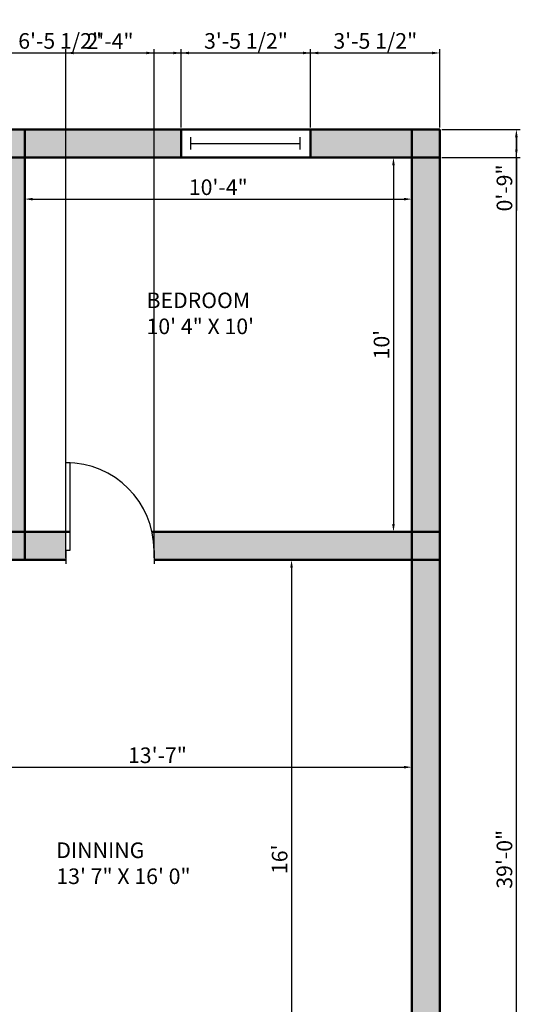
# Model space of a CAD drawing. Units: millimetres. Extents: x 2784 to 3697, y 603 to 1406.
# Tile 10 of 10: x 3537 to 3697, y 953 to 1268. Entities that reach past the tile are written whole.
import ezdxf

# ---------------------------------------------------------------- set-up
doc = ezdxf.new("R2010")
doc.units = ezdxf.units.MM
for name, color, linetype, lineweight in [('A-ANNO-DIMS', 140, 'Continuous', 18), ('A-AREA-IDEN', 150, 'Continuous', 25), ('A-DOOR', 10, 'Continuous', 25), ('A-GLAZ', 30, 'Continuous', 25), ('A-WALL', 2, 'Continuous', 50), ('A-WALL-PATT', 8, 'Continuous', 13)]:
    doc.layers.add(name, color=color, linetype=linetype, lineweight=lineweight)
doc.styles.get("Standard").update_dxf_attribs({"font": 'arial.ttf'})
doc.dimstyles.new('ISO-25', dxfattribs={"dimtxt": 5, "dimasz": 2.5, "dimexe": 1.25, "dimexo": 0.625, "dimtad": 1, "dimdec": 0, "dimlunit": 3, "dimtxsty": 'Standard', "dimcen": 2.5, "dimadec": 0, "dimazin": 0, "dimtfac": 1, "dimtdec": 0, "dimtmove": 0, "dimatfit": 3, "dimfxl": 1, "dimarcsym": 0})

# ---------------------------------------------------------------- blocks, each defined once
blk = doc.blocks.new('*U2')
for p, q in [((0, 0), (0, -6)), ((40, 0), (40, -6))]:
    blk.add_line(p, q)
blk.add_lwpolyline([(0, 0), (0, 40), (1.75, 40), (1.75, 0)], close=True)
blk.add_arc((0, 0), 40, 0, 90)
blk = doc.blocks.new('*U38')
for p, q in [((0, 4), (0, 0)), ((36, 4), (36, 0)), ((0, 2), (36, 2))]:
    blk.add_line(p, q)
blk = doc.blocks.new('*D43')
at = {"layer": 'A-ANNO-DIMS', "color": 0, "lineweight": -2, "transparency": 16777216}
for p, q in [((3661.6, 1224.28), (3655.11, 1224.28)), ((3656.36, 1221.78), (3656.36, 1106.78)), ((3661.6, 1104.28), (3655.11, 1104.28))]:
    blk.add_line(p, q, dxfattribs=at)
at = {"layer": 'A-ANNO-DIMS', "color": 0, "transparency": 16777216}
for points in [[(3655.94, 1221.78), (3656.77, 1221.78), (3656.36, 1224.28)], [(3655.94, 1106.78), (3656.77, 1106.78), (3656.36, 1104.28)]]:
    blk.add_solid(points, dxfattribs=at)
at = {"layer": 'Defpoints', "color": 0, "transparency": 16777216}
for p in [(3662.23, 1224.28), (3656.36, 1104.28), (3662.23, 1104.28)]:
    blk.add_point(p, dxfattribs=at)
at = {"layer": 'A-ANNO-DIMS', "color": 0, "transparency": 16777216, "insert": (3653.18, 1164.28), "char_height": 5, "attachment_point": 5, "rotation": 90}
blk.add_mtext("10'", dxfattribs=at)
blk = doc.blocks.new('*D44')
at = {"layer": 'A-ANNO-DIMS', "color": 0, "lineweight": -2, "transparency": 16777216}
for p, q in [((3538.23, 1211.55), (3538.23, 1212.18)), ((3662.23, 1211.55), (3662.23, 1212.18)), ((3540.73, 1210.93), (3659.73, 1210.93))]:
    blk.add_line(p, q, dxfattribs=at)
at = {"layer": 'A-ANNO-DIMS', "color": 0, "transparency": 16777216}
for points in [[(3540.73, 1211.34), (3540.73, 1210.51), (3538.23, 1210.93)], [(3659.73, 1211.34), (3659.73, 1210.51), (3662.23, 1210.93)]]:
    blk.add_solid(points, dxfattribs=at)
at = {"layer": 'Defpoints', "color": 0, "transparency": 16777216}
for p in [(3538.23, 1210.93), (3662.23, 1210.93), (3662.23, 1210.93)]:
    blk.add_point(p, dxfattribs=at)
at = {"layer": 'A-ANNO-DIMS', "color": 0, "transparency": 16777216, "insert": (3600.23, 1214.1), "char_height": 5, "attachment_point": 5}
blk.add_mtext('10\'-4"', dxfattribs=at)
blk = doc.blocks.new('*D58')
at = {"layer": 'A-ANNO-DIMS', "color": 0, "lineweight": -2, "transparency": 16777216}
for p, q in [((3624.82, 1095.28), (3622.46, 1095.28)), ((3623.71, 1092.78), (3623.71, 905.81)), ((3624.82, 903.31), (3622.46, 903.31))]:
    blk.add_line(p, q, dxfattribs=at)
at = {"layer": 'A-ANNO-DIMS', "color": 0, "transparency": 16777216}
for points in [[(3623.29, 1092.78), (3624.12, 1092.78), (3623.71, 1095.28)], [(3623.29, 905.81), (3624.12, 905.81), (3623.71, 903.31)]]:
    blk.add_solid(points, dxfattribs=at)
at = {"layer": 'Defpoints', "color": 0, "transparency": 16777216}
for p in [(3625.44, 1095.28), (3623.71, 903.31), (3625.44, 903.31)]:
    blk.add_point(p, dxfattribs=at)
at = {"layer": 'A-ANNO-DIMS', "color": 0, "transparency": 16777216, "insert": (3620.53, 999.3), "char_height": 5, "attachment_point": 5, "rotation": 90}
blk.add_mtext("16'", dxfattribs=at)
blk = doc.blocks.new('*D59')
at = {"layer": 'A-ANNO-DIMS', "color": 0, "lineweight": -2, "transparency": 16777216}
for p, q in [((3499.23, 1028.23), (3499.23, 1030.07)), ((3662.23, 1028.23), (3662.23, 1030.07)), ((3501.73, 1028.82), (3659.73, 1028.82))]:
    blk.add_line(p, q, dxfattribs=at)
at = {"layer": 'A-ANNO-DIMS', "color": 0, "transparency": 16777216}
for points in [[(3501.73, 1029.23), (3501.73, 1028.4), (3499.23, 1028.82)], [(3659.73, 1029.23), (3659.73, 1028.4), (3662.23, 1028.82)]]:
    blk.add_solid(points, dxfattribs=at)
at = {"layer": 'Defpoints', "color": 0, "transparency": 16777216}
for p in [(3499.23, 1027.6), (3662.23, 1028.82), (3662.23, 1027.6)]:
    blk.add_point(p, dxfattribs=at)
at = {"layer": 'A-ANNO-DIMS', "color": 0, "transparency": 16777216, "insert": (3580.73, 1032), "char_height": 5, "attachment_point": 5}
blk.add_mtext('13\'-7"', dxfattribs=at)
blk = doc.blocks.new('*D110')
at = {"layer": 'A-ANNO-DIMS', "color": 0, "lineweight": -2, "transparency": 16777216}
for p, q in [((3307.23, 1233.91), (3307.23, 1259.03)), ((3309.73, 1257.78), (3668.73, 1257.78)), ((3671.23, 1233.91), (3671.23, 1259.03))]:
    blk.add_line(p, q, dxfattribs=at)
at = {"layer": 'A-ANNO-DIMS', "color": 0, "transparency": 16777216}
for points in [[(3309.73, 1258.2), (3309.73, 1257.36), (3307.23, 1257.78)], [(3668.73, 1258.2), (3668.73, 1257.36), (3671.23, 1257.78)]]:
    blk.add_solid(points, dxfattribs=at)
at = {"layer": 'Defpoints', "color": 0, "transparency": 16777216}
for p in [(3671.23, 1257.78), (3307.23, 1233.28), (3671.23, 1233.28)]:
    blk.add_point(p, dxfattribs=at)
at = {"layer": 'A-ANNO-DIMS', "color": 0, "transparency": 16777216, "insert": (3489.23, 1260.96), "char_height": 5, "attachment_point": 5}
blk.add_mtext('30\'-4"', dxfattribs=at)
blk = doc.blocks.new('*D115')
at = {"layer": 'A-ANNO-DIMS', "color": 0, "lineweight": -2, "transparency": 16777216}
for p, q in [((3510.77, 1233.91), (3510.77, 1259.03)), ((3513.27, 1257.78), (3585.87, 1257.78)), ((3588.37, 1233.91), (3588.37, 1259.03))]:
    blk.add_line(p, q, dxfattribs=at)
at = {"layer": 'A-ANNO-DIMS', "color": 0, "transparency": 16777216}
for points in [[(3513.27, 1258.2), (3513.27, 1257.36), (3510.77, 1257.78)], [(3585.87, 1258.2), (3585.87, 1257.36), (3588.37, 1257.78)]]:
    blk.add_solid(points, dxfattribs=at)
at = {"layer": 'Defpoints', "color": 0, "transparency": 16777216}
for p in [(3588.37, 1257.78), (3510.77, 1233.28), (3588.37, 1233.28)]:
    blk.add_point(p, dxfattribs=at)
at = {"layer": 'A-ANNO-DIMS', "color": 0, "transparency": 16777216, "insert": (3549.57, 1260.99), "char_height": 5, "attachment_point": 5}
blk.add_mtext('6\'-5 1/2"', dxfattribs=at)
blk = doc.blocks.new('*D116')
at = {"layer": 'A-ANNO-DIMS', "color": 0, "lineweight": -2, "transparency": 16777216}
for p, q in [((3588.37, 1233.91), (3588.37, 1259.03)), ((3590.87, 1257.78), (3627.32, 1257.78)), ((3629.82, 1233.91), (3629.82, 1259.03))]:
    blk.add_line(p, q, dxfattribs=at)
at = {"layer": 'A-ANNO-DIMS', "color": 0, "transparency": 16777216}
for points in [[(3590.87, 1258.2), (3590.87, 1257.36), (3588.37, 1257.78)], [(3627.32, 1258.2), (3627.32, 1257.36), (3629.82, 1257.78)]]:
    blk.add_solid(points, dxfattribs=at)
at = {"layer": 'Defpoints', "color": 0, "transparency": 16777216}
for p in [(3629.82, 1257.78), (3588.37, 1233.28), (3629.82, 1233.28)]:
    blk.add_point(p, dxfattribs=at)
at = {"layer": 'A-ANNO-DIMS', "color": 0, "transparency": 16777216, "insert": (3609.1, 1260.99), "char_height": 5, "attachment_point": 5}
blk.add_mtext('3\'-5 1/2"', dxfattribs=at)
blk = doc.blocks.new('*D117')
at = {"layer": 'A-ANNO-DIMS', "color": 0, "lineweight": -2, "transparency": 16777216}
for p, q in [((3629.82, 1233.91), (3629.82, 1259.03)), ((3632.32, 1257.78), (3668.73, 1257.78)), ((3671.23, 1233.91), (3671.23, 1259.03))]:
    blk.add_line(p, q, dxfattribs=at)
at = {"layer": 'A-ANNO-DIMS', "color": 0, "transparency": 16777216}
for points in [[(3632.32, 1258.2), (3632.32, 1257.36), (3629.82, 1257.78)], [(3668.73, 1258.2), (3668.73, 1257.36), (3671.23, 1257.78)]]:
    blk.add_solid(points, dxfattribs=at)
at = {"layer": 'Defpoints', "color": 0, "transparency": 16777216}
for p in [(3671.23, 1257.78), (3629.82, 1233.28), (3671.23, 1233.28)]:
    blk.add_point(p, dxfattribs=at)
at = {"layer": 'A-ANNO-DIMS', "color": 0, "transparency": 16777216, "insert": (3650.53, 1260.99), "char_height": 5, "attachment_point": 5}
blk.add_mtext('3\'-5 1/2"', dxfattribs=at)
blk = doc.blocks.new('*D130')
at = {"layer": 'A-ANNO-DIMS', "color": 0, "lineweight": -2, "transparency": 16777216}
for p, q in [((3671.85, 1233.28), (3696.98, 1233.28)), ((3695.73, 767.81), (3695.73, 1230.78)), ((3671.85, 765.31), (3696.98, 765.31))]:
    blk.add_line(p, q, dxfattribs=at)
at = {"layer": 'A-ANNO-DIMS', "color": 0, "transparency": 16777216}
for points in [[(3695.31, 1230.78), (3696.14, 1230.78), (3695.73, 1233.28)], [(3695.31, 767.81), (3696.14, 767.81), (3695.73, 765.31)]]:
    blk.add_solid(points, dxfattribs=at)
at = {"layer": 'Defpoints', "color": 0, "transparency": 16777216}
for p in [(3671.23, 1233.28), (3695.73, 1233.28), (3671.23, 765.31)]:
    blk.add_point(p, dxfattribs=at)
at = {"layer": 'A-ANNO-DIMS', "color": 0, "transparency": 16777216, "insert": (3692.55, 999.3), "char_height": 5, "attachment_point": 5, "rotation": 90}
blk.add_mtext('39\'-0"', dxfattribs=at)
blk = doc.blocks.new('*D131')
at = {"layer": 'A-ANNO-DIMS', "color": 0, "lineweight": -2, "transparency": 16777216}
for p, q in [((3671.85, 1233.28), (3696.98, 1233.28)), ((3695.73, 1230.78), (3695.73, 1226.78)), ((3671.85, 1224.28), (3696.98, 1224.28)), ((3695.73, 1224.28), (3695.73, 1207.24))]:
    blk.add_line(p, q, dxfattribs=at)
at = {"layer": 'A-ANNO-DIMS', "color": 0, "transparency": 16777216}
for points in [[(3695.31, 1230.78), (3696.14, 1230.78), (3695.73, 1233.28)], [(3695.31, 1226.78), (3696.14, 1226.78), (3695.73, 1224.28)]]:
    blk.add_solid(points, dxfattribs=at)
at = {"layer": 'Defpoints', "color": 0, "transparency": 16777216}
for p in [(3671.23, 1233.28), (3671.23, 1224.28), (3695.73, 1224.28)]:
    blk.add_point(p, dxfattribs=at)
at = {"layer": 'A-ANNO-DIMS', "color": 0, "transparency": 16777216, "insert": (3692.55, 1214.51), "char_height": 5, "attachment_point": 5, "rotation": 90}
blk.add_mtext('0\'-9"', dxfattribs=at)
blk = doc.blocks.new('*D134')
at = {"layer": 'A-ANNO-DIMS', "color": 0, "lineweight": -2, "transparency": 16777216}
for p, q in [((3551.44, 1095.91), (3551.44, 1259.03)), ((3553.94, 1257.78), (3577.16, 1257.78)), ((3579.66, 1095.91), (3579.66, 1259.03))]:
    blk.add_line(p, q, dxfattribs=at)
at = {"layer": 'A-ANNO-DIMS', "color": 0, "transparency": 16777216}
for points in [[(3553.94, 1258.2), (3553.94, 1257.36), (3551.44, 1257.78)], [(3577.16, 1258.2), (3577.16, 1257.36), (3579.66, 1257.78)]]:
    blk.add_solid(points, dxfattribs=at)
at = {"layer": 'Defpoints', "color": 0, "transparency": 16777216}
for p in [(3579.66, 1257.78), (3551.44, 1095.28), (3579.66, 1095.28)]:
    blk.add_point(p, dxfattribs=at)
at = {"layer": 'A-ANNO-DIMS', "color": 0, "transparency": 16777216, "insert": (3565.55, 1260.92), "char_height": 5, "attachment_point": 5}
blk.add_mtext('2\'-4"', dxfattribs=at)

msp = doc.modelspace()

# ---------------------------------------------------------------- hatches: boundary and pattern name
at = {"layer": 'A-WALL-PATT'}
h = msp.add_hatch(color=256, dxfattribs=at)
h.dxf.hatch_style = 1
h.paths.add_polyline_path([(3316.23, 1224.28), (3307.23, 1224.28), (3307.23, 1104.28), (3316.23, 1104.28)])
h.paths.add_polyline_path([(3316.23, 1233.28), (3307.23, 1233.28), (3307.23, 1224.28), (3316.23, 1224.28)])
h.paths.add_polyline_path([(3363.37, 1233.28), (3316.23, 1233.28), (3316.23, 1224.28), (3363.37, 1224.28)])
h.paths.add_polyline_path([(3460.23, 1233.28), (3405.1, 1233.28), (3405.1, 1224.28), (3460.23, 1224.28)])
h.paths.add_polyline_path([(3469.23, 1233.28), (3460.23, 1233.28), (3460.23, 1224.28), (3469.23, 1224.28)])
h.paths.add_polyline_path([(3469.23, 1224.28), (3460.23, 1224.28), (3460.23, 1104.28), (3469.23, 1104.28)])
h.paths.add_polyline_path([(3469.23, 1104.28), (3460.23, 1104.28), (3460.23, 1095.28), (3469.23, 1095.28)])
h.paths.add_polyline_path([(3460.23, 1104.28), (3444.39, 1104.28), (3444.39, 1097.52), (3444.39, 1095.28), (3460.23, 1095.28)])
h.paths.add_polyline_path([(3409.23, 1095.28), (3400.23, 1095.28), (3400.23, 1066.17, -0.119943), (3407.82, 1068.02), (3409.23, 1068.02)])
h.paths.add_polyline_path([(3409.23, 1104.28), (3400.23, 1104.28), (3400.23, 1095.28), (3409.23, 1095.28)])
h.paths.add_polyline_path([(3400.23, 1104.28), (3316.23, 1104.28), (3316.23, 1095.28), (3400.23, 1095.28)])
h.paths.add_polyline_path([(3316.23, 1104.28), (3307.23, 1104.28), (3307.23, 1095.28), (3316.23, 1095.28)])
h.paths.add_polyline_path([(3316.23, 1095.28), (3307.23, 1095.28), (3307.23, 1083.49), (3316.23, 1083.49)])
h.paths.add_polyline_path([(3416.17, 1097.52, -0.060509), (3416.99, 1104.28), (3409.23, 1104.28), (3409.23, 1095.28), (3416.17, 1095.28)])
h.paths.add_polyline_path([(3538.23, 1224.28), (3529.23, 1224.28), (3529.23, 1104.28), (3538.23, 1104.28)])
h.paths.add_polyline_path([(3538.23, 1233.28), (3529.23, 1233.28), (3529.23, 1224.28), (3538.23, 1224.28)])
h.paths.add_polyline_path([(3529.23, 1233.28), (3510.77, 1233.28), (3510.77, 1224.28), (3529.23, 1224.28)])
h.paths.add_polyline_path([(3483.89, 1233.28), (3469.23, 1233.28), (3469.23, 1224.28), (3483.89, 1224.28)])
h.paths.add_polyline_path([(3662.23, 1233.28), (3629.82, 1233.28), (3629.82, 1224.28), (3662.23, 1224.28)])
h.paths.add_polyline_path([(3671.23, 1233.28), (3662.23, 1233.28), (3662.23, 1224.28), (3671.23, 1224.28)])
h.paths.add_polyline_path([(3671.23, 1224.28), (3662.23, 1224.28), (3662.23, 1104.28), (3671.23, 1104.28)])
h.paths.add_polyline_path([(3588.37, 1233.28), (3538.23, 1233.28), (3538.23, 1224.28), (3588.37, 1224.28)])
h.paths.add_polyline_path([(3662.23, 1104.28), (3579.01, 1104.28, -0.053945), (3579.66, 1098.24), (3579.66, 1095.28), (3662.23, 1095.28)])
h.paths.add_polyline_path([(3671.23, 1104.28), (3662.23, 1104.28), (3662.23, 1095.28), (3671.23, 1095.28)])
h.paths.add_polyline_path([(3551.44, 1104.28), (3538.23, 1104.28), (3538.23, 1095.28), (3551.44, 1095.28), (3551.44, 1098.24)])
h.paths.add_polyline_path([(3538.23, 1104.28), (3529.23, 1104.28), (3529.23, 1095.28), (3538.23, 1095.28)])
h.paths.add_polyline_path([(3671.23, 1095.28), (3662.23, 1095.28), (3662.23, 903.31), (3671.23, 903.31)])
h.paths.add_polyline_path([(3316.23, 985.84), (3307.23, 985.84), (3307.23, 932.57), (3316.23, 932.57)])
h.paths.add_polyline_path([(3316.23, 1041.28), (3307.23, 1041.28), (3307.23, 1012.14), (3316.23, 1012.14)])
h.paths.add_polyline_path([(3316.23, 1050.28), (3307.23, 1050.28), (3307.23, 1041.28), (3316.23, 1041.28)])
h.paths.add_polyline_path([(3400.23, 1050.28), (3316.23, 1050.28), (3316.23, 1041.28), (3400.23, 1041.28)])
h.paths.add_polyline_path([(3316.23, 1059.19), (3307.23, 1059.19), (3307.23, 1050.28), (3316.23, 1050.28)])
h.paths.add_polyline_path([(3316.23, 908.17), (3307.23, 908.17), (3307.23, 774.31), (3316.23, 774.31)])
h.paths.add_polyline_path([(3316.23, 774.31), (3307.23, 774.31), (3307.23, 765.31), (3316.23, 765.31)])
h.paths.add_polyline_path([(3372.55, 774.31), (3316.23, 774.31), (3316.23, 765.31), (3372.55, 765.31)])
h.paths.add_polyline_path([(3505.23, 774.31), (3416.56, 774.31), (3416.56, 765.31), (3505.23, 765.31)])
h.paths.add_polyline_path([(3568.83, 774.31), (3514.23, 774.31), (3514.23, 765.31), (3568.83, 765.31)])
h.paths.add_polyline_path([(3514.23, 774.31), (3505.23, 774.31), (3505.23, 765.31), (3514.23, 765.31)])
h.paths.add_polyline_path([(3514.23, 894.31), (3505.23, 894.31), (3505.23, 774.31), (3514.23, 774.31)])
h.paths.add_polyline_path([(3514.23, 903.31), (3505.23, 903.31), (3505.23, 894.31), (3514.23, 894.31)])
h.paths.add_polyline_path([(3473.23, 948.31), (3464.23, 948.31), (3464.23, 903.31), (3473.23, 903.31)])
h.paths.add_polyline_path([(3473.23, 903.31), (3464.23, 903.31), (3464.23, 894.31), (3473.23, 894.31)])
h.paths.add_polyline_path([(3464.23, 903.31), (3421.03, 903.31, -0.144956), (3423.7, 894.31), (3464.23, 894.31)])
h.paths.add_polyline_path([(3385.23, 903.31), (3376.23, 903.31), (3376.23, 894.31), (3385.23, 894.31)])
h.paths.add_polyline_path([(3385.23, 948.31), (3376.23, 948.31), (3376.23, 903.31), (3385.23, 903.31)])
h.paths.add_polyline_path([(3407.17, 903.31), (3385.23, 903.31), (3385.23, 894.31), (3407.17, 894.31)])
h.paths.add_polyline_path([(3353.12, 903.31), (3316.23, 903.31), (3316.23, 894.31), (3353.12, 894.31), (3353.12, 895.49)])
h.paths.add_polyline_path([(3376.23, 903.31), (3367.68, 903.31, -0.123903), (3369.65, 895.49), (3369.65, 894.31), (3376.23, 894.31)])
h.paths.add_polyline_path([(3499.23, 957.31), (3499.23, 1041.28), (3490.23, 1041.28), (3490.23, 957.31), (3316.23, 957.31), (3316.23, 948.31), (3490.23, 948.31), (3499.23, 948.31)])
h.paths.add_polyline_path([(3490.23, 1050.28), (3485.56, 1050.28), (3409.23, 1050.28), (3409.23, 1041.28), (3490.23, 1041.28)])
h.paths.add_polyline_path([(3409.23, 1050.28), (3400.23, 1050.28), (3400.23, 1041.28), (3409.23, 1041.28)])
h.paths.add_polyline_path([(3499.23, 1050.28), (3490.23, 1050.28), (3490.23, 1041.28), (3499.23, 1041.28)])
h.paths.add_polyline_path([(3671.23, 894.31), (3662.23, 894.31), (3662.23, 774.31), (3671.23, 774.31)])
h.paths.add_polyline_path([(3671.23, 903.31), (3662.23, 903.31), (3662.23, 894.31), (3671.23, 894.31)])
h.paths.add_polyline_path([(3662.23, 903.31), (3558.05, 903.31, -0.082354), (3555.98, 894.31), (3662.23, 894.31)])
h.paths.add_polyline_path([(3529.88, 903.31), (3514.23, 903.31), (3514.23, 894.31), (3529.88, 894.31)])
h.paths.add_polyline_path([(3531.12, 903.31), (3529.88, 903.31), (3529.88, 894.31), (3531.12, 894.31)])
h.paths.add_polyline_path([(3662.23, 774.31), (3610.06, 774.31), (3610.06, 765.31), (3662.23, 765.31)])
h.paths.add_polyline_path([(3671.23, 774.31), (3662.23, 774.31), (3662.23, 765.31), (3671.23, 765.31)])
h.paths.add_polyline_path([(3544.99, 801.01), (3590.84, 801.01), (3590.84, 819.67), (3544.99, 819.67)], flags=9)
h.paths.add_polyline_path([(3347.99, 824.43), (3394.58, 824.43), (3394.58, 843.09), (3347.99, 843.09)], flags=9)
h.paths.add_polyline_path([(3546.35, 988.53), (3592.21, 988.53), (3592.21, 1007.19), (3546.35, 1007.19)], flags=9)
h.paths.add_polyline_path([(3329.63, 1060.44), (3367.72, 1060.44), (3367.72, 1079.1), (3329.63, 1079.1)], flags=9)
h.paths.add_polyline_path([(3353.92, 1169.75), (3400.92, 1169.75), (3400.92, 1188.4), (3353.92, 1188.4)], flags=9)

# ---------------------------------------------------------------- linework, layer by layer
at = {"layer": 'A-WALL'}
for p, q in [((3307.23, 1233.28), (3671.23, 1233.28)), ((3538.23, 1233.28), (3538.23, 1095.28)), ((3588.37, 1233.28), (3588.37, 1224.28)), ((3629.82, 1233.28), (3629.82, 1224.28)), ((3662.23, 1233.28), (3662.23, 765.31)), ((3671.23, 1233.28), (3671.23, 765.31)), ((3307.23, 1224.28), (3671.23, 1224.28)), ((3505.25, 1104.28), (3552.67, 1104.28)), ((3579.01, 1104.28), (3671.23, 1104.28)), ((3506.8, 1095.28), (3551.44, 1095.28)), ((3579.66, 1095.28), (3671.23, 1095.28))]:
    msp.add_line(p, q, dxfattribs=at)

# ---------------------------------------------------------------- block references
at = {"layer": 'A-DOOR', "xscale": 0.7055841571326333, "yscale": 0.7055841571326333, "zscale": 0.7055841571326333}
msp.add_blockref('*U2', (3551.44, 1098.24), dxfattribs=at)
at = {"layer": 'A-GLAZ', "xscale": 0.9748873049904094, "yscale": 0.9748873049904094, "zscale": 0.9748873049904094}
msp.add_blockref('*U38', (3591.31, 1226.86), dxfattribs=at)

# ---------------------------------------------------------------- texts
at = {"layer": 'A-AREA-IDEN', "char_height": 5, "attachment_point": 1}
for s, width, insert in [('BEDROOM \\P10\' 4" X 10\'', 61.1153, (3577.25, 1180.98)), ('DINNING \\P13\' 7" X 16\' 0"', 56.269, (3548.36, 1004.7))]:
    msp.add_mtext_dynamic_manual_height_columns(s, width=width, gutter_width=12.5, heights=[0], dxfattribs=dict(at, insert=insert))

# ---------------------------------------------------------------- dimensions: what is measured, and where the dimension line sits
at = {"layer": 'A-ANNO-DIMS'}
for base, p1, p2, override, picture, middle in [((3588.37, 1257.78), (3510.77, 1233.28), (3588.37, 1233.28), {"dimdec": 1, "dimlfac": 1, "dimrnd": 0, "dimzin": 1, "dimdsep": 46, "dimlunit": 4, "dimfrac": 2}, '*D115', (3549.57, 1260.99)), ((3629.8241, 1257.7804), (3588.3666, 1233.2804), (3629.8241, 1233.2804), {"dimdec": 1, "dimlfac": 1, "dimrnd": 0, "dimzin": 1, "dimdsep": 46, "dimlunit": 4, "dimfrac": 2}, '*D116', (3609.0953, 1260.9924)), ((3671.23, 1257.78), (3629.82, 1233.28), (3671.23, 1233.28), {"dimdec": 1, "dimlfac": 1, "dimrnd": 0, "dimzin": 1, "dimdsep": 46, "dimlunit": 4, "dimfrac": 2}, '*D117', (3650.53, 1260.99)), ((3671.23, 1257.78), (3307.23, 1233.28), (3671.23, 1233.28), {"dimdec": 1, "dimlfac": 1, "dimrnd": 0, "dimzin": 1, "dimdsep": 46, "dimlunit": 4, "dimfrac": 2}, '*D110', (3489.23, 1260.96)), ((3579.66, 1257.78), (3551.44, 1095.28), (3579.66, 1095.28), {"dimdec": 1, "dimlfac": 1, "dimrnd": 0, "dimzin": 1, "dimdsep": 46, "dimlunit": 4, "dimfrac": 2}, '*D134', (3565.55, 1260.92)), ((3662.23, 1210.93), (3538.23, 1210.93), (3662.23, 1210.93), {"dimclrd": 0, "dimclre": 0, "dimclrt": 0}, '*D44', (3600.23, 1214.1)), ((3662.23, 1028.82), (3499.23, 1027.6), (3662.23, 1027.6), {"dimclrd": 0, "dimclre": 0, "dimclrt": 0}, '*D59', (3580.73, 1032))]:
    dim = msp.add_linear_dim(base=base, p1=p1, p2=p2, dimstyle='ISO-25', override=override, dxfattribs=at)
    dim.commit()
    dim.dimension.update_dxf_attribs({"geometry": picture, "text_midpoint": middle})
for base, p1, p2, override, picture, middle in [((3695.73, 1233.28), (3671.23, 765.31), (3671.23, 1233.28), {"dimdec": 1, "dimlfac": 1, "dimrnd": 0, "dimzin": 1, "dimdsep": 46, "dimlunit": 4, "dimfrac": 2}, '*D130', (3692.55, 999.3)), ((3695.73, 1224.28), (3671.23, 1233.28), (3671.23, 1224.28), {"dimdec": 1, "dimlfac": 1, "dimrnd": 0, "dimzin": 1, "dimdsep": 46, "dimlunit": 4, "dimfrac": 2}, '*D131', (3692.55, 1214.51)), ((3656.36, 1104.28), (3662.23, 1224.28), (3662.23, 1104.28), {"dimclrd": 0, "dimclre": 0, "dimclrt": 0}, '*D43', (3653.18, 1164.28)), ((3623.71, 903.31), (3625.44, 1095.28), (3625.44, 903.31), {"dimclrd": 0, "dimclre": 0, "dimclrt": 0}, '*D58', (3620.53, 999.3))]:
    dim = msp.add_linear_dim(base=base, p1=p1, p2=p2, angle=90, dimstyle='ISO-25', override=override, dxfattribs=at)
    dim.commit()
    dim.dimension.update_dxf_attribs({"geometry": picture, "text_midpoint": middle})

doc.saveas('drawing.dxf')
